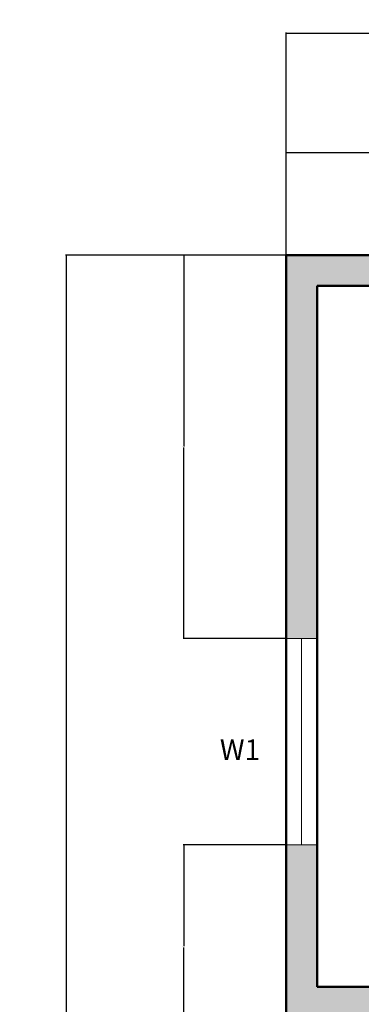
# Model space of a CAD drawing. Units: inches. Extents: x -55 to 413, y -498 to 86.
# Tile 3 of 6: x -55 to 45, y -201 to 86. Entities that reach past the tile are written whole.
import ezdxf

# ---------------------------------------------------------------- set-up
doc = ezdxf.new("R2010")
doc.units = ezdxf.units.IN
doc.header["$MEASUREMENT"] = 0
for name, color, linetype, lineweight in [('A-ANNO-DIMS', 2, 'Continuous', 18), ('A-ANNO-TEXT', 7, 'Continuous', 25), ('A-GLAZ', 4, 'Continuous', 18), ('A-WALL', 7, 'Continuous', 50), ('A-WALL-PATT', 8, 'Continuous', 13)]:
    doc.layers.add(name, color=color, linetype=linetype, lineweight=lineweight)
doc.styles.get("Standard").update_dxf_attribs({"font": 'arial.ttf'})
doc.dimstyles.get("Standard").update_dxf_attribs({"dimtxt": 0.18, "dimasz": 0.18, "dimexe": 0.18, "dimexo": 0.0625, "dimgap": 0.09, "dimtad": 0, "dimtih": 1, "dimtoh": 1, "dimdec": 0, "dimzin": 0, "dimdsep": 46, "dimlunit": 3, "dimtxsty": 'Standard', "dimcen": 0.09, "dimadec": 0, "dimazin": 0, "dimtfac": 1, "dimtdec": 0, "dimtofl": 0, "dimtmove": 0, "dimatfit": 3, "dimfxl": 1, "dimtolj": 1, "dimtzin": 0, "dimarcsym": 0})

# ---------------------------------------------------------------- blocks, each defined once
blk = doc.blocks.new('*D2')
at = {"layer": 'A-ANNO-DIMS', "color": 0, "lineweight": -2, "transparency": 16777216}
for p, q in [((23, 17.6), (23, 82.27)), ((23.18, 82.09), (197.82, 82.09)), ((382.82, 82.09), (208.18, 82.09)), ((383, 17.6), (383, 82.27))]:
    blk.add_line(p, q, dxfattribs=at)
at = {"layer": 'A-ANNO-DIMS', "color": 0, "transparency": 16777216}
for points in [[(23.18, 82.12), (23.18, 82.06), (23, 82.09)], [(382.82, 82.12), (382.82, 82.06), (383, 82.09)]]:
    blk.add_solid(points, dxfattribs=at)
at = {"layer": 'Defpoints', "color": 0, "transparency": 16777216}
for p in [(383, 82.09), (23, 17.54), (383, 17.54)]:
    blk.add_point(p, dxfattribs=at)
at = {"layer": 'A-ANNO-DIMS', "color": 0, "transparency": 16777216, "insert": (203, 82.09), "char_height": 6, "attachment_point": 5}
blk.add_mtext("\\A1;30'", dxfattribs=at)
blk = doc.blocks.new('*D3')
at = {"layer": 'A-ANNO-DIMS', "color": 0, "lineweight": -2, "transparency": 16777216}
for p, q in [((22.94, 17.54), (-41.24, 17.54)), ((-41.06, 17.36), (-41.06, -218.55)), ((-41.06, -460.78), (-41.06, -224.87)), ((22.94, -460.96), (-41.24, -460.96))]:
    blk.add_line(p, q, dxfattribs=at)
at = {"layer": 'A-ANNO-DIMS', "color": 0, "transparency": 16777216}
for points in [[(-41.09, 17.36), (-41.03, 17.36), (-41.06, 17.54)], [(-41.09, -460.78), (-41.03, -460.78), (-41.06, -460.96)]]:
    blk.add_solid(points, dxfattribs=at)
at = {"layer": 'Defpoints', "color": 0, "transparency": 16777216}
for p in [(23, 17.54), (-41.06, -460.96), (23, -460.96)]:
    blk.add_point(p, dxfattribs=at)
at = {"layer": 'A-ANNO-DIMS', "color": 0, "transparency": 16777216, "insert": (-41.06, -221.71), "char_height": 6, "attachment_point": 5}
blk.add_mtext('\\A1;39\'-11"', dxfattribs=at)
blk = doc.blocks.new('WIN-60IN')
for p, q in [((0, 9), (60, 9)), ((0, 0), (0, 9)), ((60, 9), (60, 0)), ((0, 4.5), (60, 4.5)), ((60, 0), (0, 0))]:
    blk.add_line(p, q)
blk = doc.blocks.new('*D27')
at = {"layer": 'A-ANNO-DIMS', "color": 0, "lineweight": -2, "transparency": 16777216}
for p, q in [((23, 17.6), (23, 47.52)), ((23.18, 47.34), (59.74, 47.34)), ((97.37, 47.34), (60.82, 47.34)), ((97.55, 17.6), (97.55, 47.52))]:
    blk.add_line(p, q, dxfattribs=at)
at = {"layer": 'A-ANNO-DIMS', "color": 0, "transparency": 16777216}
for points in [[(23.18, 47.37), (23.18, 47.31), (23, 47.34)], [(97.37, 47.37), (97.37, 47.31), (97.55, 47.34)]]:
    blk.add_solid(points, dxfattribs=at)
at = {"layer": 'Defpoints', "color": 0, "transparency": 16777216}
for p in [(97.55, 47.34), (23, 17.54), (97.55, 17.54)]:
    blk.add_point(p, dxfattribs=at)
at = {"layer": 'A-ANNO-DIMS', "color": 0, "transparency": 16777216, "insert": (60.28, 47.34), "char_height": 0.18, "attachment_point": 5}
blk.add_mtext('\\A1;6\'-2 1/2"', dxfattribs=at)
blk = doc.blocks.new('*D30')
at = {"layer": 'A-ANNO-DIMS', "color": 0, "lineweight": -2, "transparency": 16777216}
for p, q in [((22.94, 17.54), (-6.98, 17.54)), ((-6.8, 17.36), (-6.8, -38.09)), ((-6.8, -93.9), (-6.8, -38.45)), ((22.94, -94.08), (-6.98, -94.08))]:
    blk.add_line(p, q, dxfattribs=at)
at = {"layer": 'A-ANNO-DIMS', "color": 0, "transparency": 16777216}
for points in [[(-6.83, 17.36), (-6.77, 17.36), (-6.8, 17.54)], [(-6.83, -93.9), (-6.77, -93.9), (-6.8, -94.08)]]:
    blk.add_solid(points, dxfattribs=at)
at = {"layer": 'Defpoints', "color": 0, "transparency": 16777216}
for p in [(-6.8, 17.54), (23, 17.54), (23, -94.08)]:
    blk.add_point(p, dxfattribs=at)
at = {"layer": 'A-ANNO-DIMS', "color": 0, "transparency": 16777216, "insert": (-6.8, -38.27), "char_height": 0.18, "attachment_point": 5}
blk.add_mtext('\\A1;9\'-3 1/2"', dxfattribs=at)
blk = doc.blocks.new('*D32')
at = {"layer": 'A-ANNO-DIMS', "color": 0, "lineweight": -2, "transparency": 16777216}
for p, q in [((22.94, -154.08), (-6.98, -154.08)), ((-6.8, -154.26), (-6.8, -183.56)), ((-6.8, -213.22), (-6.8, -183.93)), ((22.94, -213.4), (-6.98, -213.4))]:
    blk.add_line(p, q, dxfattribs=at)
at = {"layer": 'A-ANNO-DIMS', "color": 0, "transparency": 16777216}
for points in [[(-6.83, -154.26), (-6.77, -154.26), (-6.8, -154.08)], [(-6.83, -213.22), (-6.77, -213.22), (-6.8, -213.4)]]:
    blk.add_solid(points, dxfattribs=at)
at = {"layer": 'Defpoints', "color": 0, "transparency": 16777216}
for p in [(23, -154.08), (-6.8, -213.4), (23, -213.4)]:
    blk.add_point(p, dxfattribs=at)
at = {"layer": 'A-ANNO-DIMS', "color": 0, "transparency": 16777216, "insert": (-6.8, -183.74), "char_height": 0.18, "attachment_point": 5}
blk.add_mtext('\\A1;4\'-11 1/2"', dxfattribs=at)

msp = doc.modelspace()

# ---------------------------------------------------------------- hatches: boundary and pattern name
at = {"layer": 'A-WALL-PATT'}
h = msp.add_hatch(color=256, dxfattribs=at)
h.dxf.hatch_style = 1
h.paths.add_polyline_path([(97.55, 17.54), (23, 17.54), (23, -94.08), (32, -94.08), (32, 8.54), (97.55, 8.54)])
h.paths.add_polyline_path([(191, 17.54), (157.55, 17.54), (157.55, 8.54), (164, 8.54), (164, -80.46), (168.5, -80.46), (173, -80.46), (173, 8.54), (191, 8.54)])
h.paths.add_polyline_path([(312.03, 17.54), (215, 17.54), (215, 8.54), (233, 8.54), (233, -111.46), (173, -111.46), (173, -108.46), (164, -108.46), (164, -164.46), (168.5, -164.46), (173, -164.46), (173, -120.46), (233, -120.46), (233, -164.46), (237.5, -164.46), (242, -164.46), (242, 8.54), (312.03, 8.54)])
h.paths.add_polyline_path([(383, 17.54), (372.03, 17.54), (372.03, 8.54), (374, 8.54), (374, -99.01), (383, -99.01)])
h.paths.add_polyline_path([(383, -159.01), (374, -159.01), (374, -195.46), (242, -195.46), (242, -192.46), (233, -192.46), (233, -204.46), (374, -204.46), (374, -224.71), (383, -224.71)])
h.paths.add_polyline_path([(173, -192.46), (164, -192.46), (164, -195.46), (32, -195.46), (32, -154.08), (23, -154.08), (23, -213.4), (32, -213.4), (32, -204.46), (164, -204.46), (164, -221.46), (168.5, -221.46), (173, -221.46)])
h.paths.add_polyline_path([(173, -249.46), (164, -249.46), (164, -252.46), (32, -252.46), (32, -237.4), (23, -237.4), (23, -273.22), (32, -273.22), (32, -261.46), (164, -261.46), (173, -261.46)])
h.paths.add_polyline_path([(32, -309.22), (23, -309.22), (23, -456.46), (23, -460.96), (199.52, -460.96), (199.52, -456.46), (32, -456.46), (32, -366.46), (97.71, -366.46), (97.71, -357.46), (32, -357.46)])
h.paths.add_polyline_path([(188.35, -357.46), (173, -357.46), (173, -302.07), (164, -302.07), (164, -357.46), (157.71, -357.46), (157.71, -366.46), (188.35, -366.46)])
h.paths.add_polyline_path([(223.25, -357.46), (212.35, -357.46), (212.35, -366.46), (223.25, -366.46), (223.25, -361.96)])
h.paths.add_polyline_path([(287.63, -357.46), (271.25, -357.46), (271.25, -361.96), (271.25, -366.46), (287.63, -366.46)])
h.paths.add_polyline_path([(374, -357.46), (311.63, -357.46), (311.63, -366.46), (374, -366.46)])
h.paths.add_polyline_path([(383, -456.46), (383, -366.46), (378.5, -366.46), (378.5, -456.46), (309.45, -456.46), (309.45, -460.96), (383, -460.96)])
h.paths.add_polyline_path([(309.45, -458.71), (199.52, -458.71), (199.52, -460.96), (309.45, -460.96)])
h.paths.add_polyline_path([(383, -260.71), (374, -260.71), (374, -280.96), (371, -280.96), (371, -285.46), (374, -285.46), (374, -366.46), (383, -366.46)])
h.paths.add_polyline_path([(343, -283.21), (343, -280.96), (321.5, -280.96), (321.5, -357.46), (326, -357.46), (326, -285.46), (343, -285.46)])

# ---------------------------------------------------------------- linework, layer by layer
at = {"layer": 'A-WALL'}
for p, q in [((23, 17.54), (23, -456.46)), ((23, 17.54), (383, 17.54)), ((32, 8.54), (164, 8.54)), ((32, 8.54), (32, -195.46)), ((32, -195.46), (164, -195.46))]:
    msp.add_line(p, q, dxfattribs=at)

# ---------------------------------------------------------------- block references
at = {"layer": 'A-GLAZ', "rotation": 90.00000000000003}
msp.add_blockref('WIN-60IN', (32, -154.08), dxfattribs=at)

# ---------------------------------------------------------------- texts
at = {"layer": 'A-ANNO-TEXT', "insert": (3.69, -123.42), "char_height": 6, "attachment_point": 1}
msp.add_mtext('W1', dxfattribs=at)

# ---------------------------------------------------------------- dimensions: what is measured, and where the dimension line sits
at = {"layer": 'A-ANNO-DIMS'}
for base, p1, p2, override, picture, middle in [((383, 82.09), (23, 17.54), (383, 17.54), {"dimtxt": 6, "dimclrd": 0, "dimclre": 0, "dimclrt": 0}, '*D2', (203, 82.09)), ((97.5535, 47.3397), (23.0027, 17.5397), (97.5535, 17.5397), {"dimdec": 1, "dimlfac": 1, "dimrnd": 0, "dimzin": 1, "dimdsep": 46, "dimlunit": 4, "dimfrac": 2}, '*D27', (60.2781, 47.3397))]:
    dim = msp.add_linear_dim(base=base, p1=p1, p2=p2, dimstyle='Standard', override=override, dxfattribs=at)
    dim.commit()
    dim.dimension.update_dxf_attribs({"geometry": picture, "text_midpoint": middle})
for base, p1, p2, override, picture, middle in [((-41.05729825, -460.96025605), (23.00267102, 17.53974395), (23.00267102, -460.96025605), {"dimtxt": 6, "dimclrd": 0, "dimclre": 0, "dimclrt": 0}, '*D3', (-41.05729825, -221.71025605)), ((-6.8, 17.54), (23, -94.08), (23, 17.54), {"dimdec": 1, "dimlfac": 1, "dimrnd": 0, "dimzin": 1, "dimdsep": 46, "dimlunit": 4, "dimfrac": 2}, '*D30', (-6.8, -38.27)), ((-6.8, -213.4), (23, -154.08), (23, -213.4), {"dimdec": 1, "dimlfac": 1, "dimrnd": 0, "dimzin": 1, "dimdsep": 46, "dimlunit": 4, "dimfrac": 2}, '*D32', (-6.8, -183.74))]:
    dim = msp.add_linear_dim(base=base, p1=p1, p2=p2, angle=90, dimstyle='Standard', override=override, dxfattribs=at)
    dim.commit()
    dim.dimension.update_dxf_attribs({"geometry": picture, "text_midpoint": middle})

doc.saveas('drawing.dxf')
